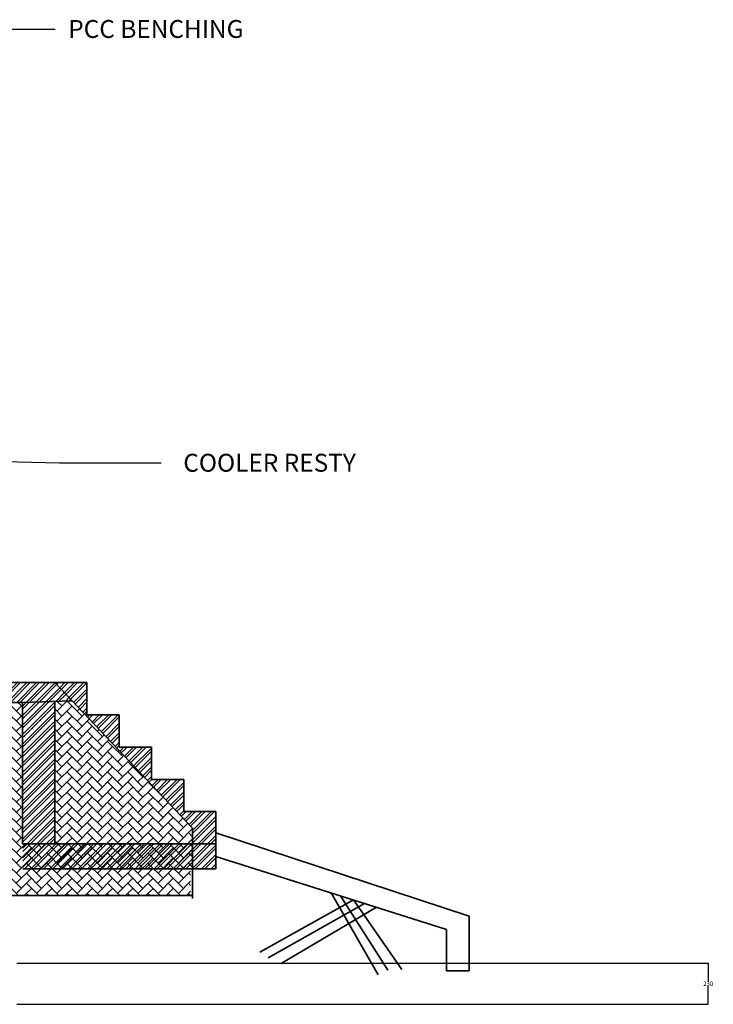
# Model space of a CAD drawing. Units: millimetres. Extents: x 1944 to 29915, y -10550 to 5909.
# Tile 21 of 24: x 26040 to 29915, y -7746 to -2251. Entities that reach past the tile are written whole.
import ezdxf
from ezdxf import colors
from ezdxf.entities.mleader import LeaderData, LeaderLine
from ezdxf.math import Vec2, Vec3

# ---------------------------------------------------------------- set-up
doc = ezdxf.new("R2010")
doc.units = ezdxf.units.MM
doc.header["$MEASUREMENT"] = 0
for name, color, linetype, lineweight in [('A-ANNO-DIMS', 2, 'Continuous', 18), ('A-ANNO-TEXT', 7, 'Continuous', 25), ('A-FLOR-PATT', 252, 'Continuous', 13), ('A-SECT', 7, 'Continuous', 35)]:
    doc.layers.add(name, color=color, linetype=linetype, lineweight=lineweight)
doc.styles.get("Standard").update_dxf_attribs({"font": 'arial.ttf'})
doc.dimstyles.get("Standard").update_dxf_attribs({"dimtxt": 25, "dimasz": 0.18, "dimexe": 0.18, "dimexo": 0.0625, "dimgap": 0.09, "dimtad": 0, "dimtih": 1, "dimtoh": 1, "dimdec": 0, "dimzin": 0, "dimdsep": 46, "dimtxsty": 'Standard', "dimcen": 0.09, "dimadec": 0, "dimazin": 0, "dimtfac": 1, "dimtdec": 0, "dimtofl": 0, "dimtmove": 0, "dimatfit": 3, "dimfxl": 1, "dimtolj": 1, "dimtzin": 0, "dimarcsym": 0})

# ---------------------------------------------------------------- blocks, each defined once
blk = doc.blocks.new('*D92')
at = {"layer": 'A-ANNO-DIMS', "color": 0, "lineweight": -2, "transparency": 16777216}
for p, q in [((26024.4, -7516.2), (29886.4, -7516.2)), ((29886.2, -7516.4), (29886.2, -7618.4)), ((29886.2, -7746), (29886.2, -7644.1)), ((26024.4, -7746.2), (29886.4, -7746.2))]:
    blk.add_line(p, q, dxfattribs=at)
at = {"layer": 'A-ANNO-DIMS', "color": 0, "transparency": 16777216}
for points in [[(29886.2, -7516.4), (29886.3, -7516.4), (29886.2, -7516.2)], [(29886.2, -7746), (29886.3, -7746), (29886.2, -7746.2)]]:
    blk.add_solid(points, dxfattribs=at)
at = {"layer": 'Defpoints', "color": 0, "transparency": 16777216}
for p in [(26024.3, -7516.2), (26024.3, -7746.2), (29886.2, -7746.2)]:
    blk.add_point(p, dxfattribs=at)
at = {"layer": 'A-ANNO-DIMS', "color": 0, "transparency": 16777216, "insert": (29886.2, -7631.2), "char_height": 25, "attachment_point": 5}
blk.add_mtext('\\A1;230', dxfattribs=at)

msp = doc.modelspace()

# ---------------------------------------------------------------- hatches: boundary and pattern name
at = {"layer": 'A-FLOR-PATT'}
h = msp.add_hatch(dxfattribs=at)
h.set_pattern_fill('ANSI32', color=256, scale=100)
h.paths.add_polyline_path([(25158.02, -5950.967), (26236.262, -5950.967), (26332.914, -6053.056), (26056.262, -6061.05), (25158.02, -6061.05)])
h = msp.add_hatch(dxfattribs=at)
h.set_pattern_fill('ANSI32', color=256, scale=100)
h.paths.add_polyline_path([(26236.262, -5950.967), (26416.262, -5950.967), (26416.262, -6130.967), (26596.262, -6130.967), (26596.262, -6310.967), (26776.262, -6310.967), (26776.262, -6490.967), (26956.262, -6490.967), (26956.262, -6670.967), (27136.262, -6670.967), (27136.262, -6850.967), (27136.262, -6990.545), (27005.891, -6990.545), (27005.891, -6763.893)], flags=17)
h = msp.add_hatch(dxfattribs=at)
h.set_pattern_fill('AR-HBONE', color=256, scale=10)
h.paths.add_polyline_path([(25389.297, -6305.752), (25389.297, -6061.05), (26056.262, -6061.05), (26056.262, -6850.967), (26236.262, -6850.967), (27005.891, -6850.967), (27005.891, -6990.545), (26995.108, -6990.545), (26995.108, -7135.877), (25389.297, -7135.877)])
h = msp.add_hatch(dxfattribs=at)
h.set_pattern_fill('ANSI32', color=256, scale=100)
h.paths.add_polyline_path([(26056.262, -6850.967), (26236.262, -6850.967), (26236.262, -6055.849), (26056.262, -6061.05)])
h = msp.add_hatch(dxfattribs=at)
h.set_pattern_fill('AR-HBONE', color=256, scale=10)
h.paths.add_polyline_path([(26236.262, -6850.967), (27005.891, -6850.967), (27005.891, -6763.893), (26332.914, -6053.056), (26236.262, -6055.849)])
h = msp.add_hatch(dxfattribs=at)
h.set_pattern_fill('ANSI32', color=256, scale=100)
h.paths.add_polyline_path([(26058.02, -6850.967), (27005.891, -6850.967), (27005.891, -6990.545), (26058.02, -6990.545)])

# ---------------------------------------------------------------- linework, layer by layer
at = {"layer": 'A-SECT'}
for p, q in [((25158.02, -5950.967), (26236.262, -5950.967)), ((26416.262, -5950.967), (26236.262, -5950.967)), ((27005.891, -6763.893), (26236.262, -5950.967)), ((26416.262, -6130.967), (26416.262, -5950.967)), ((26056.262, -6061.05), (25158.02, -6061.05)), ((26056.262, -6061.05), (26332.914, -6053.056)), ((26056.262, -6850.967), (26056.262, -6061.05)), ((26236.262, -6055.849), (26236.262, -6850.967)), ((26596.262, -6130.967), (26416.262, -6130.967)), ((26596.262, -6310.967), (26596.262, -6130.967)), ((26776.262, -6310.967), (26596.262, -6310.967)), ((26776.262, -6490.967), (26776.262, -6310.967)), ((26956.262, -6490.967), (26776.262, -6490.967)), ((26956.262, -6670.967), (26956.262, -6490.967)), ((27136.262, -6670.967), (26956.262, -6670.967)), ((27136.262, -6850.967), (27136.262, -6670.967)), ((27005.891, -6990.545), (27005.891, -6763.893)), ((27136.262, -6789.514), (28551.248, -7255.146)), ((26236.262, -6850.967), (26056.262, -6850.967)), ((27136.262, -6850.967), (26058.02, -6850.967)), ((27136.262, -6850.967), (27136.262, -6990.545)), ((28424.325, -7328.173), (27136.262, -6920.756)), ((26058.02, -6990.545), (27136.262, -6990.545)), ((27136.262, -6990.545), (27005.891, -6990.545)), ((27005.891, -6990.545), (27005.891, -7154.946)), ((27005.891, -7139.615), (25389.297, -7139.615)), ((27780.294, -7124.465), (28042.045, -7582.577)), ((27832.659, -7141.028), (28097.403, -7554.943)), ((27904.797, -7163.845), (27382.019, -7455.011)), ((27966.033, -7183.214), (27428.981, -7486.019)), ((27904.797, -7163.845), (28174.326, -7551.1)), ((28174.326, -7551.1), (27904.797, -7163.845)), ((28033.444, -7204.536), (27500.323, -7517.553)), ((28551.248, -7255.146), (28551.248, -7558.787)), ((28424.325, -7558.787), (28424.325, -7328.173)), ((28551.248, -7558.787), (28424.325, -7558.787))]:
    msp.add_line(p, q, dxfattribs=at)

# ---------------------------------------------------------------- dimensions: what is measured, and where the dimension line sits
at = {"layer": 'A-ANNO-DIMS'}
dim = msp.add_linear_dim(base=(29886.248, -7746.218), p1=(26024.297, -7516.218), p2=(26024.297, -7746.218), angle=90, dimstyle='Standard', override={"dimdec": 0, "dimlfac": 1, "dimrnd": 0, "dimzin": 0, "dimdsep": 46, "dimlunit": 2}, dxfattribs=at)
dim.commit()
dim.dimension.update_dxf_attribs({"geometry": '*D92', "text_midpoint": (29886.248, -7631.218)})

# ---------------------------------------------------------------- leaders
at = {"layer": 'A-ANNO-TEXT'}
ml = msp.add_multileader_mtext('Standard', dxfattribs=at)
ml.set_content('PCC BENCHING', color=256)
ml.set_leader_properties()
ml.build(insert=Vec2(0, 0))
ml.multileader.update_dxf_attribs({"dogleg_length": 568.936, "arrow_head_size": 100})
ctx = ml.context
ctx.base_point, ctx.char_height, ctx.arrow_head_size, ctx.landing_gap_size, ctx.plane_origin = Vec3(26238.375, -2303.899), 100, 100, 0.09, Vec3(25669.439, -2303.899)
ctx.text_align_type = 2
notes = []
notes.append((ctx, [(0, (1, 1, 0), (25669.439, -2303.899), (1, 0), 568.936, [(0, [(25253.425, -2566.843), (25356.203, -2296.612)], 0, [])])]))
ctx.mtext.insert, ctx.mtext.alignment, ctx.mtext.flow_direction = Vec3(27290.102, -2253.046), 3, 5
ml = msp.add_multileader_mtext('Standard', dxfattribs=at)
ml.set_content('COOLER RESTY', color=256)
ml.set_leader_properties()
ml.build(insert=Vec2(0, 0))
ml.multileader.update_dxf_attribs({"dogleg_length": 568.936, "arrow_head_size": 100})
ctx = ml.context
ctx.base_point, ctx.char_height, ctx.arrow_head_size, ctx.landing_gap_size, ctx.plane_origin = Vec3(26831.222, -4724.765), 100, 100, 0.09, Vec3(26262.286, -4724.765)
ctx.text_align_type = 2
notes.append((ctx, [(0, (1, 1, 0), (26262.286, -4724.765), (1, 0), 568.936, [(0, [(25846.272, -4987.709), (25949.05, -4717.477)], 0, [])])]))
ctx.mtext.insert, ctx.mtext.alignment, ctx.mtext.flow_direction = Vec3(27917.806, -4673.912), 3, 5
for ctx, leaders in notes:
    for number, flags, end, landing, length, lines in leaders:
        leader = LeaderData()
        leader.index, (leader.has_last_leader_line, leader.has_dogleg_vector, leader.attachment_direction) = number, flags
        leader.last_leader_point, leader.dogleg_vector, leader.dogleg_length = Vec3(end), Vec3(landing), length
        for number, points, colour, breaks in lines:
            line = LeaderLine()
            line.index, line.vertices, line.color, line.breaks = number, Vec3.list(points), colors.encode_raw_color(colour), breaks
            leader.lines.append(line)
        ctx.leaders.append(leader)

doc.saveas('drawing.dxf')
